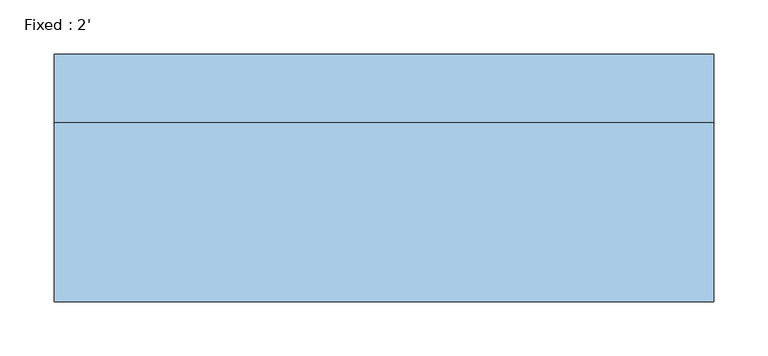
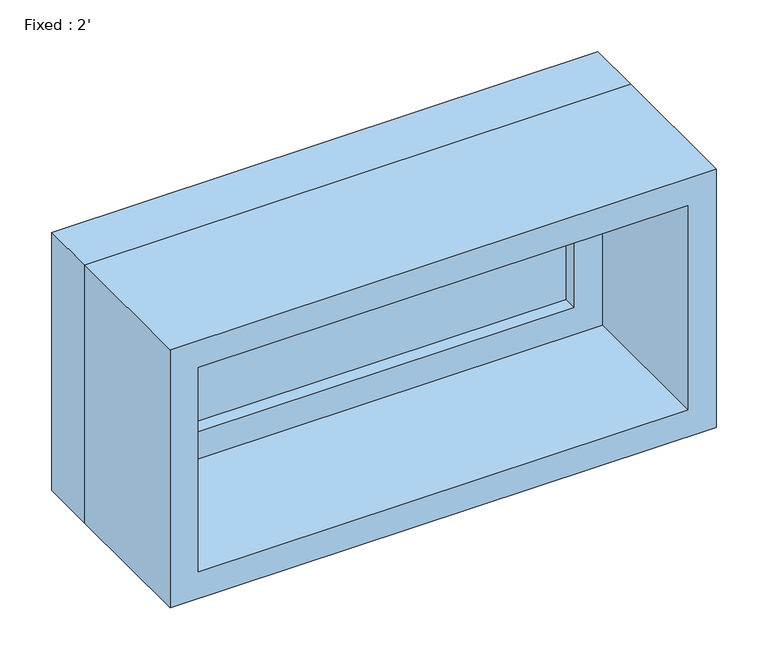
"""IFC4 building model written with IfcOpenShell, lengths in millimetres: window geometry, Fixed : 2'."""

from ifc_helpers import new_model, si_unit, frame, origin, place, context, project, spatial, polyline, outline, extrude, source, transform, mapped, element, save


def fixed_2_8c8825d0(model_context):
    return source(origin(), model_context, "Body", "SweptSolid", [
        extrude(outline(polyline([(203.2, 66.675), (-279.4, 66.675), (-279.4, 79.375), (203.2, 79.375), (203.2, 66.675)])), frame((0.0, 0.0, 977.9), z_axis=(0.0, 0.0, 1.0), x_axis=(1.0, 0.0, 0.0)), (0.0, 0.0, 1.0), 177.8),
        extrude(outline(polyline([(1200.15, -323.85), (933.45, -323.85), (933.45, 247.65), (1200.15, 247.65), (1200.15, -323.85)]), holes=[polyline([(1155.7, -279.4), (1155.7, 203.2), (977.9, 203.2), (977.9, -279.4), (1155.7, -279.4)])]), frame((0.0, 50.8, 0.0), z_axis=(0.0, 1.0, 0.0), x_axis=(0.0, 0.0, 1.0)), (0.0, 0.0, 1.0), 44.45),
        extrude(outline(polyline([(1219.2, -342.9), (914.4, -342.9), (914.4, 266.7), (1219.2, 266.7), (1219.2, -342.9)]), holes=[polyline([(1187.45, -311.15), (1187.45, 234.95), (946.15, 234.95), (946.15, -311.15), (1187.45, -311.15)])]), frame((0.0, -114.3, 0.0), z_axis=(0.0, 1.0, 0.0), x_axis=(0.0, 0.0, 1.0)), (0.0, 0.0, 1.0), 165.1),
        extrude(outline(polyline([(1219.2, 266.7), (1219.2, -342.9), (914.4, -342.9), (914.4, 266.7), (1219.2, 266.7)]), holes=[polyline([(1200.15, 247.65), (933.45, 247.65), (933.45, -323.85), (1200.15, -323.85), (1200.15, 247.65)])]), frame((0.0, 50.8, 0.0), z_axis=(0.0, 1.0, 0.0), x_axis=(0.0, 0.0, 1.0)), (0.0, 0.0, 1.0), 63.5),
    ])


if __name__ == "__main__":
    model = new_model("IFC4")
    model_context = context("Model", 3, world=origin())
    ifc_project = project(units=[si_unit("LENGTHUNIT", "METRE", prefix="MILLI")], contexts=[model_context])
    site = spatial("IfcSite", under=ifc_project)
    building = spatial("IfcBuilding", under=site)
    placement = place(None, origin())
    fixed_2_shape = fixed_2_8c8825d0(model_context)
    element("IfcWindow", 1, ObjectType="Fixed : 2'", at=placement, inside=building, context=model_context, shape_type="MappedRepresentation", body=[
        mapped(fixed_2_shape, transform((0.0, 0.0, 0.0), x_axis=(1.0, 0.0, 0.0), y_axis=(0.0, 1.0, 0.0), z_axis=(0.0, 0.0, 1.0))),
    ])
    save(model, "model.ifc")

# Revit data of these elements
# Type "Fixed : 2'"
#   Type Mark = "23"
#   Construction Type Id = "GSP4R"
#   Assembly Code = "B2020100"
#   Analytic Construction = "1/8 in Pilkington single glazing"
#   Visual Light Transmittance = 0.9
#   Solar Heat Gain Coefficient = 0.78
#   Heat Transfer Coefficient (U) = 0.6496 BTU/(h·ft²·°F)
#   Height = 1' - 0"
#   Default Sill Height = 3' - 0"
#   Width = 2' - 0"
#   Window Inset = 0' - 0 3/4"
#   Define Thermal Properties by = 1
#   Glass Pane Material = Glass
#   Sash Material = Sash
#   Wall Closure = (empty or 0)
# Element 1 (IfcWindow, "Fixed : 2'")
#   Materials on its faces: "Sash", "Glass"
# Materials
#   "Glass": class "Glass", colour RGB 0 128 192, transparency 0.75, Description = "Soda Lime Glass", Cost = 0
#   "Sash": class "Wood", colour RGB 224 178 126, transparency 0, Cost = 0
